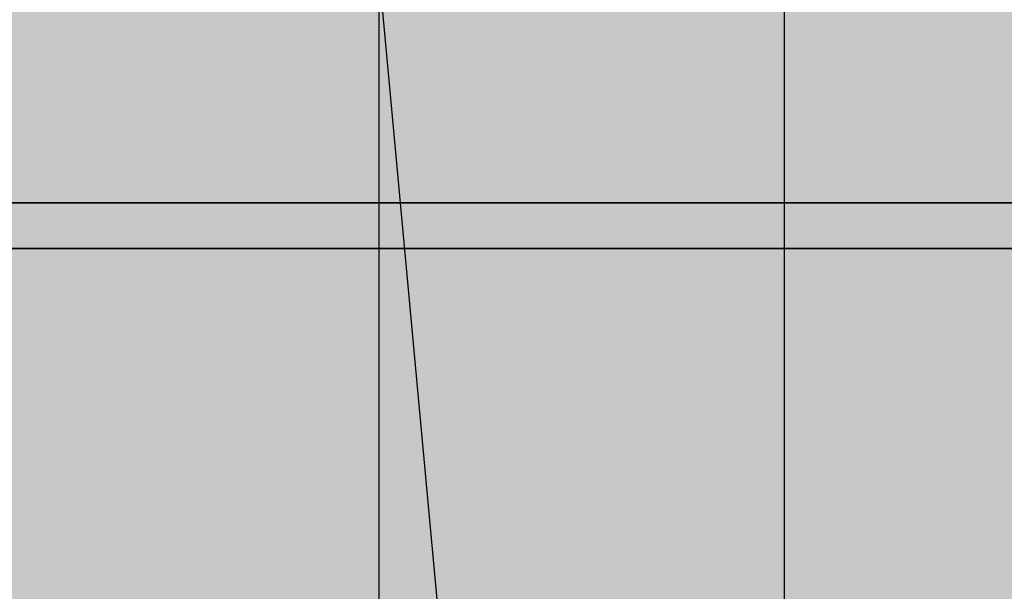
# Model space of a CAD drawing. Units: millimetres. Extents: x 130 to 1021, y 147 to 699.
# Tile 23 of 40: x 399 to 442, y 523 to 548. Entities that reach past the tile are written whole.
import ezdxf

# ---------------------------------------------------------------- set-up
doc = ezdxf.new("R2010")
doc.units = ezdxf.units.MM
doc.header["$MEASUREMENT"] = 0
for name, color, linetype, lineweight in [('A-ANNO-DIMS', 2, 'Continuous', 18), ('A-ELEV', 7, 'Continuous', 35), ('A-ELEV-PATT', 9, 'Continuous', 13)]:
    doc.layers.add(name, color=color, linetype=linetype, lineweight=lineweight)
doc.styles.get("Standard").update_dxf_attribs({"font": 'arial.ttf'})
doc.dimstyles.get("Standard").update_dxf_attribs({"dimtxt": 20, "dimasz": 10, "dimexe": 10, "dimexo": 10, "dimgap": 5, "dimtad": 0, "dimtih": 1, "dimtoh": 1, "dimdec": 0, "dimzin": 0, "dimdsep": 46, "dimtxsty": 'Standard', "dimcen": 5, "dimadec": 0, "dimazin": 0, "dimtfac": 1, "dimtdec": 0, "dimtofl": 0, "dimtmove": 0, "dimatfit": 3, "dimfxl": 1, "dimtolj": 1, "dimtzin": 0, "dimarcsym": 0})

# ---------------------------------------------------------------- blocks, each defined once
blk = doc.blocks.new('*D11')
at = {"layer": 'A-ANNO-DIMS', "color": 0, "lineweight": -2, "transparency": 16777216}
for p, q in [((737.374, 648.699), (737.374, 149.739)), ((299.374, 566.947), (299.374, 149.739)), ((309.374, 159.739), (490.857, 159.739)), ((727.374, 159.739), (545.891, 159.739))]:
    blk.add_line(p, q, dxfattribs=at)
at = {"layer": 'A-ANNO-DIMS', "color": 0, "transparency": 16777216}
for points in [[(309.374, 161.406), (309.374, 158.073), (299.374, 159.739)], [(727.374, 161.406), (727.374, 158.073), (737.374, 159.739)]]:
    blk.add_solid(points, dxfattribs=at)
at = {"layer": 'Defpoints', "color": 0, "transparency": 16777216}
for p in [(737.374, 658.699), (299.374, 576.947), (737.374, 159.739)]:
    blk.add_point(p, dxfattribs=at)
at = {"layer": 'A-ANNO-DIMS', "color": 0, "transparency": 16777216, "insert": (518.374, 159.739), "char_height": 20, "attachment_point": 5}
blk.add_mtext('\\A1;438', dxfattribs=at)
blk = doc.blocks.new('*D12')
at = {"layer": 'A-ANNO-DIMS', "color": 0, "lineweight": -2, "transparency": 16777216}
for p, q in [((477.374, 661.947), (265.074, 661.947)), ((275.074, 651.947), (275.074, 438.205)), ((275.074, 194.039), (275.074, 407.782)), ((357.163, 184.039), (265.074, 184.039))]:
    blk.add_line(p, q, dxfattribs=at)
at = {"layer": 'A-ANNO-DIMS', "color": 0, "transparency": 16777216}
for points in [[(273.407, 651.947), (276.74, 651.947), (275.074, 661.947)], [(273.407, 194.039), (276.74, 194.039), (275.074, 184.039)]]:
    blk.add_solid(points, dxfattribs=at)
at = {"layer": 'Defpoints', "color": 0, "transparency": 16777216}
for p in [(275.074, 661.947), (487.374, 661.947), (367.163, 184.039)]:
    blk.add_point(p, dxfattribs=at)
at = {"layer": 'A-ANNO-DIMS', "color": 0, "transparency": 16777216, "insert": (275.074, 422.993), "char_height": 20, "attachment_point": 5}
blk.add_mtext('\\A1;477.9', dxfattribs=at)
blk = doc.blocks.new('*D15')
at = {"layer": 'A-ANNO-DIMS', "color": 0, "lineweight": -2, "transparency": 16777216}
for p, q in [((327.374, 579.884), (327.374, 696.247)), ((357.941, 411.947), (357.941, 696.247)), ((337.374, 686.247), (347.941, 686.247)), ((357.941, 686.247), (367.941, 686.247))]:
    blk.add_line(p, q, dxfattribs=at)
at = {"layer": 'A-ANNO-DIMS', "color": 0, "transparency": 16777216}
for points in [[(337.374, 687.914), (337.374, 684.581), (327.374, 686.247)], [(347.941, 687.914), (347.941, 684.581), (357.941, 686.247)]]:
    blk.add_solid(points, dxfattribs=at)
at = {"layer": 'Defpoints', "color": 0, "transparency": 16777216}
for p in [(357.941, 686.247), (327.374, 569.884), (357.941, 401.947)]:
    blk.add_point(p, dxfattribs=at)
at = {"layer": 'A-ANNO-DIMS', "color": 0, "transparency": 16777216, "insert": (406.679, 686.247), "char_height": 20, "attachment_point": 5}
blk.add_mtext('\\A1;30.57', dxfattribs=at)
blk = doc.blocks.new('*D16')
at = {"layer": 'A-ANNO-DIMS', "color": 0, "lineweight": -2, "transparency": 16777216}
for p, q in [((357.941, 411.947), (357.941, 696.247)), ((363.922, 579.884), (363.922, 696.247)), ((347.941, 686.247), (337.941, 686.247)), ((373.922, 686.247), (383.922, 686.247))]:
    blk.add_line(p, q, dxfattribs=at)
at = {"layer": 'A-ANNO-DIMS', "color": 0, "transparency": 16777216}
for points in [[(347.941, 687.914), (347.941, 684.581), (357.941, 686.247)], [(373.922, 687.914), (373.922, 684.581), (363.922, 686.247)]]:
    blk.add_solid(points, dxfattribs=at)
at = {"layer": 'Defpoints', "color": 0, "transparency": 16777216}
for p in [(363.922, 686.247), (363.922, 569.884), (357.941, 401.947)]:
    blk.add_point(p, dxfattribs=at)
at = {"layer": 'A-ANNO-DIMS', "color": 0, "transparency": 16777216, "insert": (420.737, 686.247), "char_height": 20, "attachment_point": 5}
blk.add_mtext('\\A1;5.981', dxfattribs=at)
blk = doc.blocks.new('*D17')
at = {"layer": 'A-ANNO-DIMS', "color": 0, "lineweight": -2, "transparency": 16777216}
for p, q in [((363.922, 579.884), (363.922, 696.247)), ((375.85, 490.216), (375.85, 696.247)), ((353.922, 686.247), (343.922, 686.247)), ((385.85, 686.247), (395.85, 686.247))]:
    blk.add_line(p, q, dxfattribs=at)
at = {"layer": 'A-ANNO-DIMS', "color": 0, "transparency": 16777216}
for points in [[(353.922, 687.914), (353.922, 684.581), (363.922, 686.247)], [(385.85, 687.914), (385.85, 684.581), (375.85, 686.247)]]:
    blk.add_solid(points, dxfattribs=at)
at = {"layer": 'Defpoints', "color": 0, "transparency": 16777216}
for p in [(375.85, 686.247), (363.922, 569.884), (375.85, 480.216)]:
    blk.add_point(p, dxfattribs=at)
at = {"layer": 'A-ANNO-DIMS', "color": 0, "transparency": 16777216, "insert": (441.444, 686.247), "char_height": 20, "attachment_point": 5}
blk.add_mtext('\\A1;11.928', dxfattribs=at)
blk = doc.blocks.new('*D18')
at = {"layer": 'A-ANNO-DIMS', "color": 0, "lineweight": -2, "transparency": 16777216}
for p, q in [((375.85, 490.216), (375.85, 696.247)), ((382.374, 388.947), (382.374, 696.247)), ((365.85, 686.247), (355.85, 686.247)), ((392.374, 686.247), (402.374, 686.247))]:
    blk.add_line(p, q, dxfattribs=at)
at = {"layer": 'A-ANNO-DIMS', "color": 0, "transparency": 16777216}
for points in [[(365.85, 687.914), (365.85, 684.581), (375.85, 686.247)], [(392.374, 687.914), (392.374, 684.581), (382.374, 686.247)]]:
    blk.add_solid(points, dxfattribs=at)
at = {"layer": 'Defpoints', "color": 0, "transparency": 16777216}
for p in [(382.374, 686.247), (375.85, 480.216), (382.374, 378.947)]:
    blk.add_point(p, dxfattribs=at)
at = {"layer": 'A-ANNO-DIMS', "color": 0, "transparency": 16777216, "insert": (441.132, 686.247), "char_height": 20, "attachment_point": 5}
blk.add_mtext('\\A1;6.524', dxfattribs=at)
blk = doc.blocks.new('*D19')
at = {"layer": 'A-ANNO-DIMS', "color": 0, "lineweight": -2, "transparency": 16777216}
for p, q in [((382.374, 388.947), (382.374, 696.247)), ((414.652, 510.881), (414.652, 696.247)), ((392.374, 686.247), (404.652, 686.247)), ((414.652, 686.247), (424.652, 686.247))]:
    blk.add_line(p, q, dxfattribs=at)
at = {"layer": 'A-ANNO-DIMS', "color": 0, "transparency": 16777216}
for points in [[(392.374, 687.914), (392.374, 684.581), (382.374, 686.247)], [(404.652, 687.914), (404.652, 684.581), (414.652, 686.247)]]:
    blk.add_solid(points, dxfattribs=at)
at = {"layer": 'Defpoints', "color": 0, "transparency": 16777216}
for p in [(414.652, 686.247), (414.652, 500.881), (382.374, 378.947)]:
    blk.add_point(p, dxfattribs=at)
at = {"layer": 'A-ANNO-DIMS', "color": 0, "transparency": 16777216, "insert": (463.411, 686.247), "char_height": 20, "attachment_point": 5}
blk.add_mtext('\\A1;32.28', dxfattribs=at)
blk = doc.blocks.new('*D20')
at = {"layer": 'A-ANNO-DIMS', "color": 0, "lineweight": -2, "transparency": 16777216}
for p, q in [((414.652, 510.881), (414.652, 696.247)), ((432.374, 388.947), (432.374, 696.247)), ((404.652, 686.247), (394.652, 686.247)), ((442.374, 686.247), (452.374, 686.247))]:
    blk.add_line(p, q, dxfattribs=at)
at = {"layer": 'A-ANNO-DIMS', "color": 0, "transparency": 16777216}
for points in [[(404.652, 687.914), (404.652, 684.581), (414.652, 686.247)], [(442.374, 687.914), (442.374, 684.581), (432.374, 686.247)]]:
    blk.add_solid(points, dxfattribs=at)
at = {"layer": 'Defpoints', "color": 0, "transparency": 16777216}
for p in [(432.374, 686.247), (414.652, 500.881), (432.374, 378.947)]:
    blk.add_point(p, dxfattribs=at)
at = {"layer": 'A-ANNO-DIMS', "color": 0, "transparency": 16777216, "insert": (490.075, 686.247), "char_height": 20, "attachment_point": 5}
blk.add_mtext('\\A1;17.72', dxfattribs=at)
blk = doc.blocks.new('*D21')
at = {"layer": 'A-ANNO-DIMS', "color": 0, "lineweight": -2, "transparency": 16777216}
for p, q in [((432.374, 388.947), (432.374, 696.247)), ((447.374, 656.947), (447.374, 696.247)), ((422.374, 686.247), (412.374, 686.247)), ((457.374, 686.247), (467.374, 686.247))]:
    blk.add_line(p, q, dxfattribs=at)
at = {"layer": 'A-ANNO-DIMS', "color": 0, "transparency": 16777216}
for points in [[(422.374, 687.914), (422.374, 684.581), (432.374, 686.247)], [(457.374, 687.914), (457.374, 684.581), (447.374, 686.247)]]:
    blk.add_solid(points, dxfattribs=at)
at = {"layer": 'Defpoints', "color": 0, "transparency": 16777216}
for p in [(447.374, 686.247), (447.374, 646.947), (432.374, 378.947)]:
    blk.add_point(p, dxfattribs=at)
at = {"layer": 'A-ANNO-DIMS', "color": 0, "transparency": 16777216, "insert": (485.832, 686.247), "char_height": 20, "attachment_point": 5}
blk.add_mtext('\\A1;15', dxfattribs=at)
blk = doc.blocks.new('*D22')
at = {"layer": 'A-ANNO-DIMS', "color": 0, "lineweight": -2, "transparency": 16777216}
for p, q in [((447.374, 656.947), (447.374, 696.247)), ((466.767, 403.947), (466.767, 696.247)), ((437.374, 686.247), (427.374, 686.247)), ((476.767, 686.247), (486.767, 686.247))]:
    blk.add_line(p, q, dxfattribs=at)
at = {"layer": 'A-ANNO-DIMS', "color": 0, "transparency": 16777216}
for points in [[(437.374, 687.914), (437.374, 684.581), (447.374, 686.247)], [(476.767, 687.914), (476.767, 684.581), (466.767, 686.247)]]:
    blk.add_solid(points, dxfattribs=at)
at = {"layer": 'Defpoints', "color": 0, "transparency": 16777216}
for p in [(466.767, 686.247), (447.374, 646.947), (466.767, 393.947)]:
    blk.add_point(p, dxfattribs=at)
at = {"layer": 'A-ANNO-DIMS', "color": 0, "transparency": 16777216, "insert": (532.34, 686.247), "char_height": 20, "attachment_point": 5}
blk.add_mtext('\\A1;19.393', dxfattribs=at)
blk = doc.blocks.new('*D43')
at = {"layer": 'A-ANNO-DIMS', "color": 0, "lineweight": -2, "transparency": 16777216}
for p, q in [((275.074, 510.881), (275.074, 520.881)), ((275.074, 520.881), (285.074, 520.881)), ((404.652, 500.881), (265.074, 500.881)), ((317.374, 480.95), (265.074, 480.95)), ((275.074, 470.95), (275.074, 460.95))]:
    blk.add_line(p, q, dxfattribs=at)
at = {"layer": 'A-ANNO-DIMS', "color": 0, "transparency": 16777216}
for points in [[(273.407, 510.881), (276.74, 510.881), (275.074, 500.881)], [(273.407, 470.95), (276.74, 470.95), (275.074, 480.95)]]:
    blk.add_solid(points, dxfattribs=at)
at = {"layer": 'Defpoints', "color": 0, "transparency": 16777216}
for p in [(275.074, 500.881), (414.652, 500.881), (327.374, 480.95)]:
    blk.add_point(p, dxfattribs=at)
at = {"layer": 'A-ANNO-DIMS', "color": 0, "transparency": 16777216, "insert": (322.877, 520.881), "char_height": 20, "attachment_point": 5}
blk.add_mtext('\\A1;19.93', dxfattribs=at)
blk = doc.blocks.new('*D44')
at = {"layer": 'A-ANNO-DIMS', "color": 0, "lineweight": -2, "transparency": 16777216}
for p, q in [((317.374, 569.884), (265.074, 569.884)), ((275.074, 559.884), (275.074, 550.594)), ((275.074, 510.881), (275.074, 520.171)), ((404.652, 500.881), (265.074, 500.881))]:
    blk.add_line(p, q, dxfattribs=at)
at = {"layer": 'A-ANNO-DIMS', "color": 0, "transparency": 16777216}
for points in [[(273.407, 559.884), (276.74, 559.884), (275.074, 569.884)], [(273.407, 510.881), (276.74, 510.881), (275.074, 500.881)]]:
    blk.add_solid(points, dxfattribs=at)
at = {"layer": 'Defpoints', "color": 0, "transparency": 16777216}
for p in [(275.074, 569.884), (327.374, 569.884), (414.652, 500.881)]:
    blk.add_point(p, dxfattribs=at)
at = {"layer": 'A-ANNO-DIMS', "color": 0, "transparency": 16777216, "insert": (275.074, 535.383), "char_height": 20, "attachment_point": 5}
blk.add_mtext('\\A1;69', dxfattribs=at)
blk = doc.blocks.new('*D66')
at = {"layer": 'A-ANNO-DIMS', "color": 0, "lineweight": -2, "transparency": 16777216}
for p, q in [((341.579, 557.194), (351.579, 557.194)), ((351.579, 557.194), (376.947, 478.135)), ((427.374, 315.978), (427.374, 325.978)), ((422.374, 320.978), (432.374, 320.978))]:
    blk.add_line(p, q, dxfattribs=at)
at = {"layer": 'A-ANNO-DIMS', "color": 0, "transparency": 16777216}
blk.add_solid([(378.534, 478.644), (375.36, 477.626), (380.002, 468.613)], dxfattribs=at)
at = {"layer": 'Defpoints', "color": 0, "transparency": 16777216}
for p in [(380.002, 468.613), (427.374, 320.978)]:
    blk.add_point(p, dxfattribs=at)
at = {"layer": 'A-ANNO-DIMS', "color": 0, "transparency": 16777216, "insert": (263.53, 557.194), "char_height": 20, "attachment_point": 5}
blk.add_mtext('\\A1;4X R155.05', dxfattribs=at)
blk = doc.blocks.new('*D68')
at = {"layer": 'A-ANNO-DIMS', "color": 0, "lineweight": -2, "transparency": 16777216}
for p, q in [((361.841, 579.756), (371.841, 579.756)), ((371.841, 579.756), (392.167, 506.693)), ((433.191, 354.23), (433.191, 364.23)), ((428.191, 359.23), (438.191, 359.23))]:
    blk.add_line(p, q, dxfattribs=at)
at = {"layer": 'A-ANNO-DIMS', "color": 0, "transparency": 16777216}
blk.add_solid([(393.773, 507.14), (390.561, 506.246), (394.847, 497.059)], dxfattribs=at)
at = {"layer": 'Defpoints', "color": 0, "transparency": 16777216}
for p in [(394.847, 497.059), (433.191, 359.23)]:
    blk.add_point(p, dxfattribs=at)
at = {"layer": 'A-ANNO-DIMS', "color": 0, "transparency": 16777216, "insert": (305.764, 579.756), "char_height": 20, "attachment_point": 5}
blk.add_mtext('\\A1;R143.06', dxfattribs=at)
blk = doc.blocks.new('*D69')
at = {"layer": 'A-ANNO-DIMS', "color": 0, "lineweight": -2, "transparency": 16777216}
for p, q in [((507.746, 572.261), (483.091, 501.813)), ((517.746, 572.261), (507.746, 572.261)), ((433.191, 354.23), (433.191, 364.23)), ((428.191, 359.23), (438.191, 359.23))]:
    blk.add_line(p, q, dxfattribs=at)
at = {"layer": 'A-ANNO-DIMS', "color": 0, "transparency": 16777216}
blk.add_solid([(481.518, 502.363), (484.664, 501.262), (479.788, 492.374)], dxfattribs=at)
at = {"layer": 'Defpoints', "color": 0, "transparency": 16777216}
for p in [(479.788, 492.374), (433.191, 359.23)]:
    blk.add_point(p, dxfattribs=at)
at = {"layer": 'A-ANNO-DIMS', "color": 0, "transparency": 16777216, "insert": (573.824, 572.261), "char_height": 20, "attachment_point": 5}
blk.add_mtext('\\A1;R141.06', dxfattribs=at)
blk = doc.blocks.new('*D70')
at = {"layer": 'A-ANNO-DIMS', "color": 0, "lineweight": -2, "transparency": 16777216}
for p, q in [((370.141, 588.4), (380.141, 588.4)), ((380.141, 588.4), (397.473, 517.008)), ((432.65, 367.109), (432.65, 377.109)), ((427.65, 372.109), (437.65, 372.109))]:
    blk.add_line(p, q, dxfattribs=at)
at = {"layer": 'A-ANNO-DIMS', "color": 0, "transparency": 16777216}
blk.add_solid([(399.093, 517.402), (395.854, 516.615), (399.832, 507.291)], dxfattribs=at)
at = {"layer": 'Defpoints', "color": 0, "transparency": 16777216}
for p in [(399.832, 507.291), (432.65, 372.109)]:
    blk.add_point(p, dxfattribs=at)
at = {"layer": 'A-ANNO-DIMS', "color": 0, "transparency": 16777216, "insert": (323.757, 588.4), "char_height": 20, "attachment_point": 5}
blk.add_mtext('\\A1;R139.1', dxfattribs=at)
blk = doc.blocks.new('*D71')
at = {"layer": 'A-ANNO-DIMS', "color": 0, "lineweight": -2, "transparency": 16777216}
for p, q in [((492.108, 581.609), (472.542, 512.666)), ((502.108, 581.609), (492.108, 581.609)), ((432.65, 367.109), (432.65, 377.109)), ((427.65, 372.109), (437.65, 372.109))]:
    blk.add_line(p, q, dxfattribs=at)
at = {"layer": 'A-ANNO-DIMS', "color": 0, "transparency": 16777216}
blk.add_solid([(470.938, 513.121), (474.145, 512.211), (469.812, 503.046)], dxfattribs=at)
at = {"layer": 'Defpoints', "color": 0, "transparency": 16777216}
for p in [(469.812, 503.046), (432.65, 372.109)]:
    blk.add_point(p, dxfattribs=at)
at = {"layer": 'A-ANNO-DIMS', "color": 0, "transparency": 16777216, "insert": (548.493, 581.609), "char_height": 20, "attachment_point": 5}
blk.add_mtext('\\A1;R136.1', dxfattribs=at)
blk = doc.blocks.new('*D72')
at = {"layer": 'A-ANNO-DIMS', "color": 0, "lineweight": -2, "transparency": 16777216}
for p, q in [((460.658, 573.64), (451.279, 503.49)), ((470.658, 573.64), (460.658, 573.64)), ((432.115, 355.142), (432.115, 365.142)), ((427.115, 360.142), (437.115, 360.142))]:
    blk.add_line(p, q, dxfattribs=at)
at = {"layer": 'A-ANNO-DIMS', "color": 0, "transparency": 16777216}
blk.add_solid([(449.628, 503.711), (452.931, 503.27), (449.954, 493.579)], dxfattribs=at)
at = {"layer": 'Defpoints', "color": 0, "transparency": 16777216}
for p in [(449.954, 493.579), (432.115, 360.142)]:
    blk.add_point(p, dxfattribs=at)
at = {"layer": 'A-ANNO-DIMS', "color": 0, "transparency": 16777216, "insert": (526.64, 573.64), "char_height": 20, "attachment_point": 5}
blk.add_mtext('\\A1;R134.62', dxfattribs=at)
blk = doc.blocks.new('*D73')
at = {"layer": 'A-ANNO-DIMS', "color": 0, "lineweight": -2, "transparency": 16777216}
for p, q in [((402.678, 571.448), (412.678, 571.448)), ((412.678, 571.448), (419.051, 502.166)), ((432.115, 355.142), (432.115, 365.142)), ((427.115, 360.142), (437.115, 360.142))]:
    blk.add_line(p, q, dxfattribs=at)
at = {"layer": 'A-ANNO-DIMS', "color": 0, "transparency": 16777216}
blk.add_solid([(420.711, 502.319), (417.391, 502.014), (419.967, 492.208)], dxfattribs=at)
at = {"layer": 'Defpoints', "color": 0, "transparency": 16777216}
for p in [(419.967, 492.208), (432.115, 360.142)]:
    blk.add_point(p, dxfattribs=at)
at = {"layer": 'A-ANNO-DIMS', "color": 0, "transparency": 16777216, "insert": (346.696, 571.448), "char_height": 20, "attachment_point": 5}
blk.add_mtext('\\A1;R132.62', dxfattribs=at)

msp = doc.modelspace()

# ---------------------------------------------------------------- hatches: boundary and pattern name
at = {"layer": 'A-ELEV-PATT'}
h = msp.add_hatch(color=256, dxfattribs=at)
h.dxf.hatch_style = 1
h.paths.add_polyline_path([(737.3738, 658.6988, 0.0135961), (632.4019, 661.9473), (607.3738, 661.9473), (487.3738, 661.9473), (487.3738, 649.9473), (607.3738, 649.9473), (632.3794, 649.9473, -0.0136841), (737.3738, 646.6784)])
h.paths.add_polyline_path([(732.3738, 643.9599, 0.0130529), (632.3738, 646.9473), (607.3738, 646.9473), (487.3738, 646.9473), (487.3738, 596.9473), (632.3738, 596.9473, -0.0130529), (732.3738, 593.9599)])
h.paths.add_polyline_path([(737.3738, 593.6732, 0.0137063), (632.3738, 596.9473), (487.3738, 596.9473), (487.3738, 586.9473), (632.355, 586.9473, -0.0137808), (737.3738, 583.6559)])
h.paths.add_polyline_path([(447.3738, 646.9473), (307.3738, 646.9473), (302.3738, 646.9473), (302.3738, 634.9473), (447.3738, 634.9473)])
h.paths.add_polyline_path([(447.3738, 631.9473), (307.3738, 631.9473), (307.3738, 586.9473), (447.3738, 586.9473)])
h.paths.add_polyline_path([(447.3738, 586.9473), (307.3738, 586.9473), (302.3738, 586.9473), (302.3738, 576.9473), (447.3738, 576.9473)])
h.paths.add_polyline_path([(447.3738, 573.9473), (367.3738, 573.9473), (367.3738, 539.9473), (447.3738, 539.9473)])
h.paths.add_polyline_path([(447.3738, 537.9473), (367.3738, 537.9473), (367.3738, 507.9473), (400.392, 507.4253, -0.001728), (401.3281, 507.6451, -0.5220025), (425.6117, 511.0391, -0.0391849), (447.3738, 510.4359), (447.3738, 510.7883)])
h.paths.add_polyline_path([(394.7238, 505.9473), (367.3738, 505.9473), (367.3738, 476.9473, -0.0146512), (375.8501, 480.2159), (376.1506, 499.2266, -0.0355419)])
h.paths.add_polyline_path([(632.3738, 583.9473), (552.3738, 583.9473), (552.3738, 550.9473), (632.3738, 550.9473)])
h.paths.add_polyline_path([(632.3738, 548.9473), (552.3738, 548.9473), (552.3738, 515.9473), (632.3738, 515.9473)])
h.paths.add_polyline_path([(632.3738, 513.9473), (552.3738, 513.9473), (552.3738, 476.9473), (632.3738, 476.9473)])
h.paths.add_polyline_path([(737.3738, 473.6903, 0.0136326), (632.3926, 476.9473), (552.3738, 476.9473), (487.3738, 476.9473), (487.3738, 466.9473), (632.3738, 466.9473, -0.0137063), (737.3738, 463.6732)])
h.paths.add_polyline_path([(732.3738, 460.9552, 0.0130741), (632.3681, 463.9473), (487.3738, 463.9473), (487.3738, 407.735, -0.0032286), (489.3544, 406.9473), (632.3926, 406.9473, -0.0129826), (732.3738, 403.9755)])
h.paths.add_polyline_path([(487.3738, 463.9473, 0.20133), (367.3738, 463.9473), (367.3738, 407.735, -0.1882031), (487.3738, 407.735)])
h.paths.add_polyline_path([(367.3738, 476.9473), (367.3738, 466.9473, -0.2013309), (487.3738, 466.9473), (487.3738, 476.9473, 0.20133)])
h.paths.add_polyline_path([(367.3738, 463.9473), (307.3738, 463.9473), (307.3738, 401.9473), (357.9413, 401.9473), (367.3738, 407.735)])
h.paths.add_polyline_path([(367.3738, 476.9473), (302.3738, 476.9473), (302.3738, 466.9473), (367.3738, 466.9473)])
h.paths.add_polyline_path([(632.8184, 366.9453), (552.3738, 366.9453), (552.3738, 393.9473), (632.8184, 393.9473)])
h.paths.add_polyline_path([(632.8184, 357.2114), (632.8184, 363.9453), (552.3738, 363.9453), (552.3738, 357.2114), (552.3738, 336.9453), (632.8184, 336.9453)])
h.paths.add_polyline_path([(632.8184, 333.9453), (552.3738, 333.9453), (552.3738, 306.9453), (632.8184, 306.9453)])
h.paths.add_polyline_path([(632.8184, 303.9453), (552.3738, 303.9453), (552.3738, 273.9473), (632.355, 273.9473, 0.0000608), (632.8184, 273.9491)])
h.paths.add_polyline_path([(737.3738, 403.6903, 0.0136326), (632.3926, 406.9473), (489.3544, 406.9473, 0.1915481), (367.3738, 407.735), (367.3738, 396.9473, -0.2013309), (487.3738, 396.9473), (632.3738, 396.9473, -0.0137063), (737.3738, 393.6732)])
h.paths.add_polyline_path([(357.9413, 401.9473), (307.3738, 401.9473), (307.3738, 391.9473), (357.9413, 391.9473)])
h.paths.add_polyline_path([(357.9413, 357.2114), (357.9413, 388.9473), (307.3738, 388.9473), (307.3738, 357.2114), (307.3738, 273.9473), (357.9413, 273.9473)])
h.paths.add_polyline_path([(732.3738, 263.93, -0.0130317), (632.3794, 260.9473), (466.7667, 260.9473), (466.7667, 240.9473), (469.8406, 236.978), (469.8406, 221.978), (472.9145, 218.0087), (472.9145, 213.9473), (607.3738, 213.9473), (732.3738, 213.9473)])
h.paths.add_polyline_path([(732.3738, 290.889), (722.479, 290.889), (722.479, 301.889), (732.3738, 301.889), (732.3738, 305.889), (722.479, 305.889), (722.479, 316.889), (732.3738, 316.889), (732.3738, 320.889), (722.479, 320.889), (722.479, 331.889), (732.3738, 331.889), (732.3738, 335.889), (722.479, 335.889), (722.479, 346.889), (732.3738, 346.889), (732.3738, 350.889), (722.479, 350.889), (722.479, 361.889), (732.3738, 361.889), (732.3738, 365.889), (722.479, 365.889), (722.479, 376.889), (732.3738, 376.889), (732.3738, 380.889), (722.479, 380.889), (722.479, 391.4848, 0.0005233), (718.479, 391.6843), (718.479, 380.889), (707.479, 380.889), (707.479, 392.1896, 0.0005231), (703.479, 392.3576), (703.479, 380.889), (692.479, 380.889), (692.479, 392.7765, 0.0005229), (688.479, 392.9131), (688.479, 380.889), (677.479, 380.889), (677.479, 393.2456, 0.0005228), (673.479, 393.3508), (673.479, 380.889), (662.479, 380.889), (662.479, 393.597, 0.0005227), (658.479, 393.6709), (658.479, 380.889), (647.479, 380.889), (647.479, 393.8308, 0.0005226), (643.479, 393.8732), (643.479, 380.889), (632.8184, 380.889), (632.8184, 376.889), (643.479, 376.889), (643.479, 365.889), (632.8184, 365.889), (632.8184, 361.889), (643.479, 361.889), (643.479, 350.889), (632.8184, 350.889), (632.8184, 346.889), (643.479, 346.889), (643.479, 335.889), (632.8184, 335.889), (632.8184, 331.889), (643.479, 331.889), (643.479, 320.889), (632.8184, 320.889), (632.8184, 316.889), (643.479, 316.889), (643.479, 305.889), (632.8184, 305.889), (632.8184, 301.889), (643.479, 301.889), (643.479, 290.889), (632.8184, 290.889), (632.8184, 286.889), (643.479, 286.889), (643.479, 274.0217, 0.0005246), (647.479, 274.0643), (647.479, 286.889), (658.479, 286.889), (658.479, 274.2248, 0.0005246), (662.479, 274.2989), (662.479, 286.889), (673.479, 286.889), (673.479, 274.546, 0.0005247), (677.479, 274.6516), (677.479, 286.889), (688.479, 286.889), (688.479, 274.9853, 0.0005248), (692.479, 275.1224), (692.479, 286.889), (703.479, 286.889), (703.479, 275.5429, 0.000525), (707.479, 275.7115), (707.479, 286.889), (718.479, 286.889), (718.479, 276.2187, 0.0005252), (722.479, 276.4189), (722.479, 286.889), (732.3738, 286.889)])
h.paths.add_polyline_path([(718.479, 290.889), (707.479, 290.889), (707.479, 301.889), (718.479, 301.889)], flags=16)
h.paths.add_polyline_path([(703.479, 290.889), (692.479, 290.889), (692.479, 301.889), (703.479, 301.889)], flags=16)
h.paths.add_polyline_path([(718.479, 305.889), (707.479, 305.889), (707.479, 316.889), (718.479, 316.889)], flags=16)
h.paths.add_polyline_path([(703.479, 305.889), (692.479, 305.889), (692.479, 316.889), (703.479, 316.889)], flags=16)
h.paths.add_polyline_path([(688.479, 290.889), (677.479, 290.889), (677.479, 301.889), (688.479, 301.889)], flags=16)
h.paths.add_polyline_path([(718.479, 320.889), (707.479, 320.889), (707.479, 331.889), (718.479, 331.889)], flags=16)
h.paths.add_polyline_path([(688.479, 305.889), (677.479, 305.889), (677.479, 316.889), (688.479, 316.889)], flags=16)
h.paths.add_polyline_path([(703.479, 320.889), (692.479, 320.889), (692.479, 331.889), (703.479, 331.889)], flags=16)
h.paths.add_polyline_path([(688.479, 320.889), (677.479, 320.889), (677.479, 331.889), (688.479, 331.889)], flags=16)
h.paths.add_polyline_path([(673.479, 290.889), (662.479, 290.889), (662.479, 301.889), (673.479, 301.889)], flags=16)
h.paths.add_polyline_path([(718.479, 335.889), (707.479, 335.889), (707.479, 346.889), (718.479, 346.889)], flags=16)
h.paths.add_polyline_path([(673.479, 305.889), (662.479, 305.889), (662.479, 316.889), (673.479, 316.889)], flags=16)
h.paths.add_polyline_path([(703.479, 335.889), (692.479, 335.889), (692.479, 346.889), (703.479, 346.889)], flags=16)
h.paths.add_polyline_path([(673.479, 320.889), (662.479, 320.889), (662.479, 331.889), (673.479, 331.889)], flags=16)
h.paths.add_polyline_path([(688.479, 335.889), (677.479, 335.889), (677.479, 346.889), (688.479, 346.889)], flags=16)
h.paths.add_polyline_path([(658.479, 290.889), (647.479, 290.889), (647.479, 301.889), (658.479, 301.889)], flags=16)
h.paths.add_polyline_path([(718.479, 350.889), (707.479, 350.889), (707.479, 361.889), (718.479, 361.889)], flags=16)
h.paths.add_polyline_path([(658.479, 305.889), (647.479, 305.889), (647.479, 316.889), (658.479, 316.889)], flags=16)
h.paths.add_polyline_path([(703.479, 350.889), (692.479, 350.889), (692.479, 361.889), (703.479, 361.889)], flags=16)
h.paths.add_polyline_path([(673.479, 335.889), (662.479, 335.889), (662.479, 346.889), (673.479, 346.889)], flags=16)
h.paths.add_polyline_path([(658.479, 320.889), (647.479, 320.889), (647.479, 331.889), (658.479, 331.889)], flags=16)
h.paths.add_polyline_path([(688.479, 350.889), (677.479, 350.889), (677.479, 361.889), (688.479, 361.889)], flags=16)
h.paths.add_polyline_path([(718.479, 365.889), (707.479, 365.889), (707.479, 376.889), (718.479, 376.889)], flags=16)
h.paths.add_polyline_path([(658.479, 335.889), (647.479, 335.889), (647.479, 346.889), (658.479, 346.889)], flags=16)
h.paths.add_polyline_path([(673.479, 350.889), (662.479, 350.889), (662.479, 361.889), (673.479, 361.889)], flags=16)
h.paths.add_polyline_path([(703.479, 365.889), (692.479, 365.889), (692.479, 376.889), (703.479, 376.889)], flags=16)
h.paths.add_polyline_path([(688.479, 365.889), (677.479, 365.889), (677.479, 376.889), (688.479, 376.889)], flags=16)
h.paths.add_polyline_path([(658.479, 350.889), (647.479, 350.889), (647.479, 361.889), (658.479, 361.889)], flags=16)
h.paths.add_polyline_path([(673.479, 365.889), (662.479, 365.889), (662.479, 376.889), (673.479, 376.889)], flags=16)
h.paths.add_polyline_path([(658.479, 365.889), (647.479, 365.889), (647.479, 376.889), (658.479, 376.889)], flags=16)
h.paths.add_polyline_path([(732.3738, 503.9786), (722.3392, 503.9786), (722.3392, 514.9786), (732.3738, 514.9786), (732.3738, 518.9786), (722.3392, 518.9786), (722.3392, 529.9786), (732.3738, 529.9786), (732.3738, 533.9786), (722.3392, 533.9786), (722.3392, 544.9786), (732.3738, 544.9786), (732.3738, 546.9473), (732.3738, 548.9786), (722.3392, 548.9786), (722.3392, 559.9786), (732.3738, 559.9786), (732.3738, 563.9786), (722.3392, 563.9786), (722.3392, 574.9786), (732.3738, 574.9786), (732.3738, 578.9786), (722.3392, 578.9786), (722.3392, 581.4789, 0.000526), (718.3392, 581.6791), (718.3392, 578.9786), (707.3392, 578.9786), (707.3392, 582.1863, 0.0005258), (703.3392, 582.355), (703.3392, 578.9786), (692.3392, 578.9786), (692.3392, 582.7752, 0.0005257), (688.3392, 582.9123), (688.3392, 578.9786), (677.3392, 578.9786), (677.3392, 583.2457, 0.0005255), (673.3392, 583.3512), (673.3392, 578.9786), (662.3392, 578.9786), (662.3392, 583.5978, 0.0005254), (658.3392, 583.6718), (658.3392, 578.9786), (647.3392, 578.9786), (647.3392, 583.8317, 0.0005254), (643.3392, 583.8741), (643.3392, 578.9786), (632.3738, 578.9786), (632.3738, 574.9786), (643.3392, 574.9786), (643.3392, 563.9786), (632.3738, 563.9786), (632.3738, 559.9786), (643.3392, 559.9786), (643.3392, 548.9786), (632.3738, 548.9786), (632.3738, 544.9786), (643.3392, 544.9786), (643.3392, 533.9786), (632.3738, 533.9786), (632.3738, 529.9786), (643.3392, 529.9786), (643.3392, 518.9786), (632.3738, 518.9786), (632.3738, 515.9473), (632.3738, 514.9786), (643.3392, 514.9786), (643.3392, 503.9786), (632.3738, 503.9786), (632.3738, 499.9786), (643.3392, 499.9786), (643.3392, 488.9786), (632.3738, 488.9786), (632.3738, 484.9786), (643.3392, 484.9786), (643.3392, 476.8751, -0.0005191), (647.3392, 476.8332), (647.3392, 484.9786), (658.3392, 484.9786), (658.3392, 476.6752, -0.0005192), (662.3392, 476.6022), (662.3392, 484.9786), (673.3392, 484.9786), (673.3392, 476.3585, -0.0005193), (677.3392, 476.2543), (677.3392, 484.9786), (688.3392, 484.9786), (688.3392, 475.9248, -0.0005194), (692.3392, 475.7894), (692.3392, 484.9786), (703.3392, 484.9786), (703.3392, 475.3741, -0.0005195), (707.3392, 475.2075), (707.3392, 484.9786), (718.3392, 484.9786), (718.3392, 474.7064, -0.0005197), (722.3392, 474.5086), (722.3392, 484.9786), (732.3738, 484.9786), (732.3738, 488.9786), (722.3392, 488.9786), (722.3392, 499.9786), (732.3738, 499.9786)])
h.paths.add_polyline_path([(718.3392, 503.9786), (707.3392, 503.9786), (707.3392, 514.9786), (718.3392, 514.9786)], flags=16)
h.paths.add_polyline_path([(718.3392, 499.9786), (718.3392, 488.9786), (707.3392, 488.9786), (707.3392, 499.9786)], flags=16)
h.paths.add_polyline_path([(718.3392, 518.9786), (707.3392, 518.9786), (707.3392, 529.9786), (718.3392, 529.9786)], flags=16)
h.paths.add_polyline_path([(703.3392, 503.9786), (692.3392, 503.9786), (692.3392, 514.9786), (703.3392, 514.9786)], flags=16)
h.paths.add_polyline_path([(703.3392, 499.9786), (703.3392, 488.9786), (692.3392, 488.9786), (692.3392, 499.9786)], flags=16)
h.paths.add_polyline_path([(703.3392, 518.9786), (692.3392, 518.9786), (692.3392, 529.9786), (703.3392, 529.9786)], flags=16)
h.paths.add_polyline_path([(718.3392, 533.9786), (707.3392, 533.9786), (707.3392, 544.9786), (718.3392, 544.9786)], flags=16)
h.paths.add_polyline_path([(688.3392, 503.9786), (677.3392, 503.9786), (677.3392, 514.9786), (688.3392, 514.9786)], flags=16)
h.paths.add_polyline_path([(688.3392, 499.9786), (688.3392, 488.9786), (677.3392, 488.9786), (677.3392, 499.9786)], flags=16)
h.paths.add_polyline_path([(703.3392, 533.9786), (692.3392, 533.9786), (692.3392, 544.9786), (703.3392, 544.9786)], flags=16)
h.paths.add_polyline_path([(688.3392, 518.9786), (677.3392, 518.9786), (677.3392, 529.9786), (688.3392, 529.9786)], flags=16)
h.paths.add_polyline_path([(688.3392, 533.9786), (677.3392, 533.9786), (677.3392, 544.9786), (688.3392, 544.9786)], flags=16)
h.paths.add_polyline_path([(718.3392, 548.9786), (707.3392, 548.9786), (707.3392, 559.9786), (718.3392, 559.9786)], flags=16)
h.paths.add_polyline_path([(673.3392, 503.9786), (662.3392, 503.9786), (662.3392, 514.9786), (673.3392, 514.9786)], flags=16)
h.paths.add_polyline_path([(673.3392, 499.9786), (673.3392, 488.9786), (662.3392, 488.9786), (662.3392, 499.9786)], flags=16)
h.paths.add_polyline_path([(703.3392, 548.9786), (692.3392, 548.9786), (692.3392, 559.9786), (703.3392, 559.9786)], flags=16)
h.paths.add_polyline_path([(673.3392, 518.9786), (662.3392, 518.9786), (662.3392, 529.9786), (673.3392, 529.9786)], flags=16)
h.paths.add_polyline_path([(688.3392, 548.9786), (677.3392, 548.9786), (677.3392, 559.9786), (688.3392, 559.9786)], flags=16)
h.paths.add_polyline_path([(673.3392, 533.9786), (662.3392, 533.9786), (662.3392, 544.9786), (673.3392, 544.9786)], flags=16)
h.paths.add_polyline_path([(718.3392, 563.9786), (707.3392, 563.9786), (707.3392, 574.9786), (718.3392, 574.9786)], flags=16)
h.paths.add_polyline_path([(658.3392, 503.9786), (647.3392, 503.9786), (647.3392, 514.9786), (658.3392, 514.9786)], flags=16)
h.paths.add_polyline_path([(658.3392, 499.9786), (658.3392, 488.9786), (647.3392, 488.9786), (647.3392, 499.9786)], flags=16)
h.paths.add_polyline_path([(703.3392, 563.9786), (692.3392, 563.9786), (692.3392, 574.9786), (703.3392, 574.9786)], flags=16)
h.paths.add_polyline_path([(658.3392, 518.9786), (647.3392, 518.9786), (647.3392, 529.9786), (658.3392, 529.9786)], flags=16)
h.paths.add_polyline_path([(673.3392, 548.9786), (662.3392, 548.9786), (662.3392, 559.9786), (673.3392, 559.9786)], flags=16)
h.paths.add_polyline_path([(688.3392, 563.9786), (677.3392, 563.9786), (677.3392, 574.9786), (688.3392, 574.9786)], flags=16)
h.paths.add_polyline_path([(658.3392, 533.9786), (647.3392, 533.9786), (647.3392, 544.9786), (658.3392, 544.9786)], flags=16)
h.paths.add_polyline_path([(673.3392, 563.9786), (662.3392, 563.9786), (662.3392, 574.9786), (673.3392, 574.9786)], flags=16)
h.paths.add_polyline_path([(658.3392, 548.9786), (647.3392, 548.9786), (647.3392, 559.9786), (658.3392, 559.9786)], flags=16)
h.paths.add_polyline_path([(658.3392, 563.9786), (647.3392, 563.9786), (647.3392, 574.9786), (658.3392, 574.9786)], flags=16)
h = msp.add_hatch(color=256, dxfattribs=at)
h.dxf.hatch_style = 1
h.paths.add_polyline_path([(447.3738, 537.9473), (447.3738, 539.9473), (367.3738, 539.9473), (367.3738, 537.9473)])
h.paths.add_polyline_path([(394.7238, 505.9473, -0.0105284), (400.392, 507.4253), (367.3738, 507.9473), (367.3738, 505.9473)])
h.paths.add_polyline_path([(547.7773, 546.9473), (547.7773, 548.9473), (502.3738, 548.9473), (502.3738, 546.9473)])
h.paths.add_polyline_path([(632.3738, 548.9473), (632.3738, 550.9473), (552.3738, 550.9473), (552.3738, 548.9473)])
h.paths.add_polyline_path([(632.3738, 513.9473), (632.3738, 515.9473), (552.3738, 515.9473), (552.3738, 513.9473)])
h.paths.add_polyline_path([(544.6354, 360.9453), (544.6354, 363.9453), (486.7667, 363.9454), (486.7667, 360.9454)])
h.paths.add_polyline_path([(632.8184, 363.9453), (632.8184, 366.9453), (552.3738, 366.9453), (552.3738, 363.9453)])
h.paths.add_polyline_path([(632.8184, 333.9453), (632.8184, 336.9453), (552.3738, 336.9453), (552.3738, 333.9453)])
h.paths.add_polyline_path([(552.3738, 306.9453), (552.3738, 303.9453), (632.8184, 303.9453), (632.8184, 306.9453)])

# ---------------------------------------------------------------- linework, layer by layer
at = {"layer": 'A-ELEV'}
for p, q in [((367.3738, 539.9473), (447.3738, 539.9473)), ((367.3738, 537.9473), (447.3738, 537.9473))]:
    msp.add_line(p, q, dxfattribs=at)

# ---------------------------------------------------------------- dimensions: what is measured, and where the dimension line sits
at = {"layer": 'A-ANNO-DIMS'}
for base, p1, p2, override, picture, middle in [((357.9413, 686.2473), (327.3738, 569.884), (357.9413, 401.9473), {"dimdec": 2, "dimlfac": 1, "dimrnd": 0, "dimzin": 0, "dimdsep": 46, "dimlunit": 2}, '*D15', (406.6794, 686.2473)), ((363.922, 686.2473), (357.9413, 401.9473), (363.922, 569.884), {"dimdec": 3, "dimlfac": 1, "dimrnd": 0, "dimzin": 0, "dimdsep": 46, "dimlunit": 2}, '*D16', (420.7365, 686.2473)), ((375.8501, 686.2473), (363.922, 569.884), (375.8501, 480.2159), {"dimdec": 3, "dimlfac": 1, "dimrnd": 0, "dimzin": 0, "dimdsep": 46, "dimlunit": 2}, '*D17', (441.4435, 686.2473)), ((382.3738, 686.2473), (375.8501, 480.2159), (382.3738, 378.9473), {"dimdec": 3, "dimlfac": 1, "dimrnd": 0, "dimzin": 0, "dimdsep": 46, "dimlunit": 2}, '*D18', (441.1323, 686.2473)), ((414.6525, 686.2473), (382.3738, 378.9473), (414.6525, 500.8811), {"dimdec": 2, "dimlfac": 1, "dimrnd": 0, "dimzin": 0, "dimdsep": 46, "dimlunit": 2}, '*D19', (463.411, 686.2473)), ((432.3738, 686.2473), (414.6525, 500.8811), (432.3738, 378.9473), {"dimdec": 2, "dimlfac": 1, "dimrnd": 0, "dimzin": 0, "dimdsep": 46, "dimlunit": 2}, '*D20', (490.075, 686.2473)), ((447.3738, 686.2473), (432.3738, 378.9473), (447.3738, 646.9473), {"dimdec": 0, "dimlfac": 1, "dimrnd": 0, "dimzin": 0, "dimdsep": 46, "dimlunit": 2}, '*D21', (485.8322, 686.2473)), ((466.7667, 686.2473), (447.3738, 646.9473), (466.7667, 393.9473), {"dimdec": 3, "dimlfac": 1, "dimrnd": 0, "dimzin": 0, "dimdsep": 46, "dimlunit": 2}, '*D22', (532.3397, 686.2473)), ((737.3738, 159.7395), (299.3738, 576.9473), (737.3738, 658.6988), {"dimdec": 0, "dimlfac": 1, "dimrnd": 0, "dimzin": 0, "dimdsep": 46, "dimlunit": 2}, '*D11', (518.3738, 159.7395))]:
    dim = msp.add_linear_dim(base=base, p1=p1, p2=p2, dimstyle='Standard', override=override, dxfattribs=at)
    dim.commit()
    dim.dimension.update_dxf_attribs({"geometry": picture, "text_midpoint": middle})
for base, p1, p2, override, picture, middle in [((275.0738, 661.9473), (367.163, 184.0395), (487.3738, 661.9473), {"dimdec": 1, "dimlfac": 1, "dimrnd": 0, "dimzin": 0, "dimdsep": 46, "dimlunit": 2}, '*D12', (275.0738, 422.9934)), ((275.0738, 569.884), (414.6525, 500.8811), (327.3738, 569.884), {"dimdec": 0, "dimlfac": 1, "dimrnd": 0, "dimzin": 0, "dimdsep": 46, "dimlunit": 2}, '*D44', (275.0738, 535.3826)), ((275.0738, 500.8811), (327.3738, 480.95), (414.6525, 500.8811), {"dimdec": 2, "dimlfac": 1, "dimrnd": 0, "dimzin": 0, "dimdsep": 46, "dimlunit": 2}, '*D43', (322.8773, 520.8811))]:
    dim = msp.add_linear_dim(base=base, p1=p1, p2=p2, angle=90, dimstyle='Standard', override=override, dxfattribs=at)
    dim.commit()
    dim.dimension.update_dxf_attribs({"geometry": picture, "text_midpoint": middle})
for center, mpoint, override, picture, middle in [((432.6505, 372.1087), (399.8323, 507.2907), {"dimdec": 1, "dimlfac": 1, "dimrnd": 0, "dimzin": 0, "dimdsep": 46, "dimlunit": 2}, '*D70', (323.7567, 588.3999)), ((432.6505, 372.1087), (469.8116, 503.0461), {"dimdec": 1, "dimlfac": 1, "dimrnd": 0, "dimzin": 0, "dimdsep": 46, "dimlunit": 2}, '*D71', (548.493, 581.6085)), ((433.1906, 359.2304), (394.8473, 497.0587), {"dimdec": 2, "dimlfac": 1, "dimrnd": 0, "dimzin": 0, "dimdsep": 46, "dimlunit": 2}, '*D68', (305.7636, 579.7557)), ((432.115, 360.1423), (449.9544, 493.5786), {"dimdec": 2, "dimlfac": 1, "dimrnd": 0, "dimzin": 0, "dimdsep": 46, "dimlunit": 2}, '*D72', (526.6403, 573.6404)), ((433.1906, 359.2304), (479.788, 492.3743), {"dimdec": 2, "dimlfac": 1, "dimrnd": 0, "dimzin": 0, "dimdsep": 46, "dimlunit": 2}, '*D69', (573.8242, 572.2606)), ((432.115, 360.1423), (419.967, 492.2083), {"dimdec": 2, "dimlfac": 1, "dimrnd": 0, "dimzin": 0, "dimdsep": 46, "dimlunit": 2}, '*D73', (346.696, 571.4479))]:
    dim = msp.add_radius_dim(center=center, mpoint=mpoint, dimstyle='Standard', override=override, dxfattribs=at)
    dim.commit()
    dim.dimension.update_dxf_attribs({"geometry": picture, "text_midpoint": middle, "dimtype": 164})
dim = msp.add_radius_dim(center=(427.3738, 320.9781), mpoint=(380.0022, 468.6132), text='4X <>', dimstyle='Standard', override={"dimdec": 2, "dimlfac": 1, "dimrnd": 0, "dimzin": 0, "dimdsep": 46, "dimlunit": 2}, dxfattribs=at)
dim.commit()
dim.dimension.update_dxf_attribs({"geometry": '*D66', "text_midpoint": (263.5301, 557.1943), "dimtype": 164})

doc.saveas('drawing.dxf')
